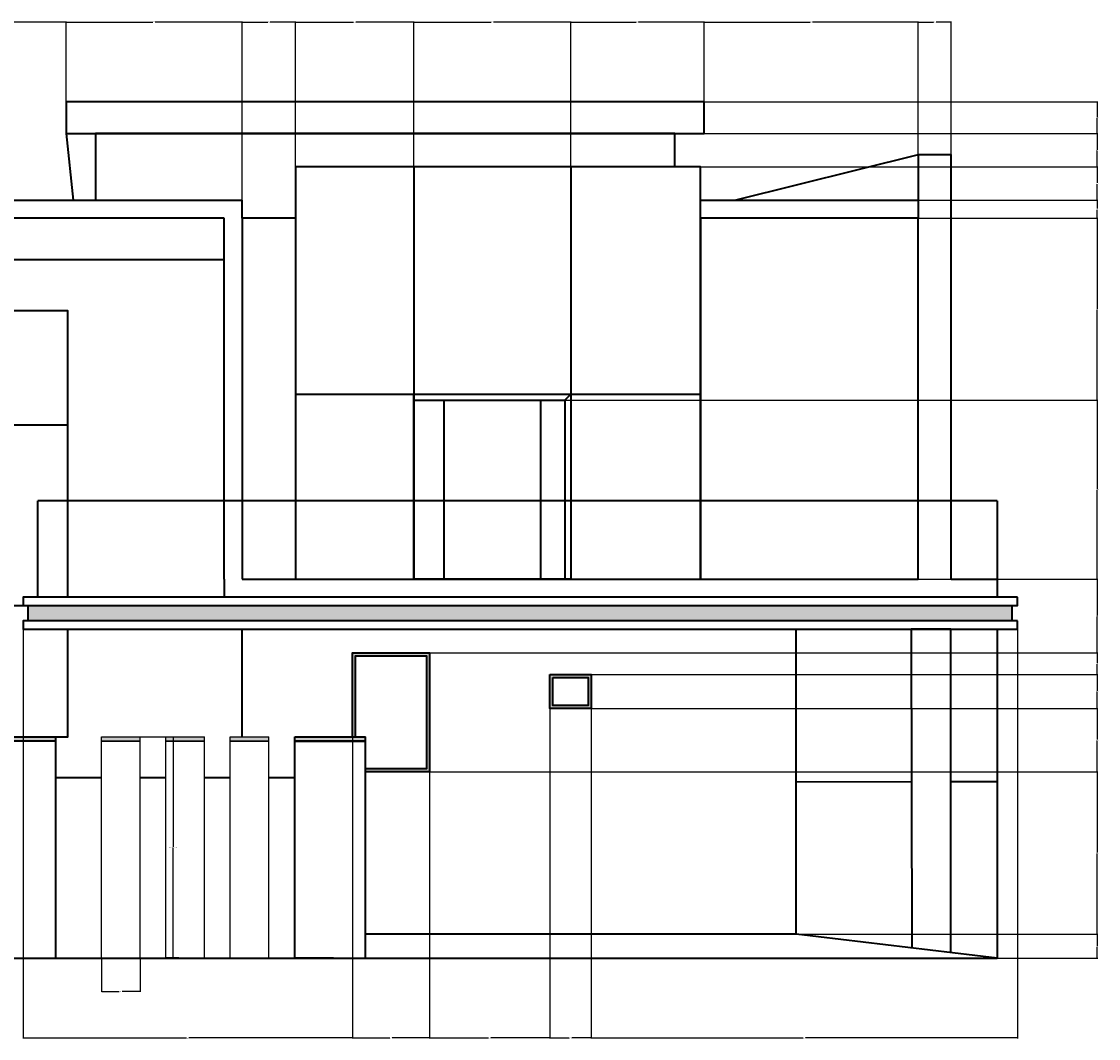
# Model space of a CAD drawing. Units: feet. Extents: x 2651 to 4047, y 949 to 1287.
# Tile 5 of 5: x 3689 to 4047, y 949 to 1287. Entities that reach past the tile are written whole.
import ezdxf

# ---------------------------------------------------------------- set-up
doc = ezdxf.new("R2010")
doc.units = ezdxf.units.FT
for name, color, linetype, lineweight in [('A-ANNO-DIMS', 2, 'Continuous', 18), ('A-ELEV', 7, 'Continuous', 35), ('A-ELEV-FNCE', 7, 'Continuous', 25), ('A-ELEV-PATT', 8, 'Continuous', 13)]:
    doc.layers.add(name, color=color, linetype=linetype, lineweight=lineweight)
doc.styles.get("Standard").update_dxf_attribs({"font": 'arial.ttf'})
doc.dimstyles.get("Standard").update_dxf_attribs({"dimtxt": 0.18, "dimasz": 0.18, "dimexe": 0.18, "dimexo": 0.0625, "dimgap": 0.09, "dimtad": 0, "dimtih": 1, "dimtoh": 1, "dimdec": 1, "dimzin": 0, "dimdsep": 46, "dimlunit": 3, "dimtxsty": 'Standard', "dimcen": 0.09, "dimadec": 0, "dimazin": 0, "dimtfac": 1, "dimtdec": 1, "dimtofl": 0, "dimtmove": 0, "dimatfit": 3, "dimfxl": 1, "dimtolj": 1, "dimtzin": 0, "dimarcsym": 0})

# ---------------------------------------------------------------- blocks, each defined once
blk = doc.blocks.new('BOUNDARY-PIER')
for p, q in [((0, 72.1), (0, 73.54)), ((12.86, 0), (12.86, 73.54))]:
    blk.add_line(p, q)
for points in [[(0, 73.54), (12.86, 73.54)], [(12.86, 0), (0, 0), (0, 72.1), (12.86, 72.1)], [(12.86, 72.1), (0, 72.1)]]:
    blk.add_lwpolyline(points)
blk = doc.blocks.new('*D5')
at = {"layer": 'A-ANNO-DIMS', "color": 0, "lineweight": -2, "transparency": 16777216}
for p, q in [((3728.81, 1049.19), (3739.96, 1049.19)), ((3739.78, 1049.01), (3739.78, 1012.6)), ((3739.78, 975.83), (3739.78, 1012.23)), ((3728.81, 975.65), (3739.96, 975.65))]:
    blk.add_line(p, q, dxfattribs=at)
at = {"layer": 'A-ANNO-DIMS', "color": 0, "transparency": 16777216}
for points in [[(3739.75, 1049.01), (3739.81, 1049.01), (3739.78, 1049.19)], [(3739.75, 975.83), (3739.81, 975.83), (3739.78, 975.65)]]:
    blk.add_solid(points, dxfattribs=at)
at = {"layer": 'Defpoints', "color": 0, "transparency": 16777216}
for p in [(3728.75, 1049.19), (3739.78, 1049.19), (3728.75, 975.65)]:
    blk.add_point(p, dxfattribs=at)
at = {"layer": 'A-ANNO-DIMS', "color": 0, "transparency": 16777216, "insert": (3739.78, 1012.42), "char_height": 0.18, "attachment_point": 5}
blk.add_mtext('\\A1;BOUNDARY PIER 74 TYP.', dxfattribs=at)
blk = doc.blocks.new('*D6')
at = {"layer": 'A-ANNO-DIMS', "color": 0, "lineweight": -2, "transparency": 16777216}
for p, q in [((3715.89, 975.59), (3715.89, 964.44)), ((3728.75, 975.59), (3728.75, 964.44)), ((3716.07, 964.62), (3721.8, 964.62)), ((3728.57, 964.62), (3722.84, 964.62))]:
    blk.add_line(p, q, dxfattribs=at)
at = {"layer": 'A-ANNO-DIMS', "color": 0, "transparency": 16777216}
for points in [[(3716.07, 964.65), (3716.07, 964.59), (3715.89, 964.62)], [(3728.57, 964.65), (3728.57, 964.59), (3728.75, 964.62)]]:
    blk.add_solid(points, dxfattribs=at)
at = {"layer": 'Defpoints', "color": 0, "transparency": 16777216}
for p in [(3715.89, 975.65), (3728.75, 975.65), (3728.75, 964.62)]:
    blk.add_point(p, dxfattribs=at)
at = {"layer": 'A-ANNO-DIMS', "color": 0, "transparency": 16777216, "insert": (3722.32, 964.62), "char_height": 0.18, "attachment_point": 5}
blk.add_mtext('\\A1;13 TYP.', dxfattribs=at)
blk = doc.blocks.new('*D30')
at = {"layer": 'A-ANNO-DIMS', "color": 0, "lineweight": -2, "transparency": 16777216}
for p, q in [((3655.82, 1190.93), (3655.82, 1287.01)), ((3656, 1286.83), (3679.52, 1286.83)), ((3703.97, 1286.83), (3680.45, 1286.83)), ((3704.15, 1260.39), (3704.15, 1287.01))]:
    blk.add_line(p, q, dxfattribs=at)
at = {"layer": 'A-ANNO-DIMS', "color": 0, "transparency": 16777216}
for points in [[(3656, 1286.86), (3656, 1286.8), (3655.82, 1286.83)], [(3703.97, 1286.86), (3703.97, 1286.8), (3704.15, 1286.83)]]:
    blk.add_solid(points, dxfattribs=at)
at = {"layer": 'Defpoints', "color": 0, "transparency": 16777216}
for p in [(3704.15, 1286.83), (3704.15, 1260.33), (3655.82, 1190.87)]:
    blk.add_point(p, dxfattribs=at)
at = {"layer": 'A-ANNO-DIMS', "color": 0, "transparency": 16777216, "insert": (3679.99, 1286.83), "char_height": 0.18, "attachment_point": 5}
blk.add_mtext('\\A1;48.335', dxfattribs=at)
blk = doc.blocks.new('*D31')
at = {"layer": 'A-ANNO-DIMS', "color": 0, "lineweight": -2, "transparency": 16777216}
for p, q in [((3704.15, 1260.39), (3704.15, 1287.01)), ((3704.33, 1286.83), (3733.04, 1286.83)), ((3762.53, 1286.83), (3733.83, 1286.83)), ((3762.71, 1227.71), (3762.71, 1287.01))]:
    blk.add_line(p, q, dxfattribs=at)
at = {"layer": 'A-ANNO-DIMS', "color": 0, "transparency": 16777216}
for points in [[(3704.33, 1286.86), (3704.33, 1286.8), (3704.15, 1286.83)], [(3762.53, 1286.86), (3762.53, 1286.8), (3762.71, 1286.83)]]:
    blk.add_solid(points, dxfattribs=at)
at = {"layer": 'Defpoints', "color": 0, "transparency": 16777216}
for p in [(3762.71, 1286.83), (3704.15, 1260.33), (3762.71, 1227.65)]:
    blk.add_point(p, dxfattribs=at)
at = {"layer": 'A-ANNO-DIMS', "color": 0, "transparency": 16777216, "insert": (3733.43, 1286.83), "char_height": 0.18, "attachment_point": 5}
blk.add_mtext('\\A1;58.56', dxfattribs=at)
blk = doc.blocks.new('*D32')
at = {"layer": 'A-ANNO-DIMS', "color": 0, "lineweight": -2, "transparency": 16777216}
for p, q in [((3762.71, 1227.71), (3762.71, 1287.01)), ((3762.89, 1286.83), (3771.2, 1286.83)), ((3780.27, 1286.83), (3771.97, 1286.83)), ((3780.45, 1238.76), (3780.45, 1287.01))]:
    blk.add_line(p, q, dxfattribs=at)
at = {"layer": 'A-ANNO-DIMS', "color": 0, "transparency": 16777216}
for points in [[(3762.89, 1286.86), (3762.89, 1286.8), (3762.71, 1286.83)], [(3780.27, 1286.86), (3780.27, 1286.8), (3780.45, 1286.83)]]:
    blk.add_solid(points, dxfattribs=at)
at = {"layer": 'Defpoints', "color": 0, "transparency": 16777216}
for p in [(3780.45, 1286.83), (3780.45, 1238.69), (3762.71, 1227.65)]:
    blk.add_point(p, dxfattribs=at)
at = {"layer": 'A-ANNO-DIMS', "color": 0, "transparency": 16777216, "insert": (3771.58, 1286.83), "char_height": 0.18, "attachment_point": 5}
blk.add_mtext('\\A1;17.74', dxfattribs=at)
blk = doc.blocks.new('*D33')
at = {"layer": 'A-ANNO-DIMS', "color": 0, "lineweight": -2, "transparency": 16777216}
for p, q in [((3780.45, 1238.76), (3780.45, 1287.01)), ((3780.63, 1286.83), (3799.7, 1286.83)), ((3819.56, 1286.83), (3800.49, 1286.83)), ((3819.74, 1238.76), (3819.74, 1287.01))]:
    blk.add_line(p, q, dxfattribs=at)
at = {"layer": 'A-ANNO-DIMS', "color": 0, "transparency": 16777216}
for points in [[(3780.63, 1286.86), (3780.63, 1286.8), (3780.45, 1286.83)], [(3819.56, 1286.86), (3819.56, 1286.8), (3819.74, 1286.83)]]:
    blk.add_solid(points, dxfattribs=at)
at = {"layer": 'Defpoints', "color": 0, "transparency": 16777216}
for p in [(3819.74, 1286.83), (3780.45, 1238.69), (3819.74, 1238.69)]:
    blk.add_point(p, dxfattribs=at)
at = {"layer": 'A-ANNO-DIMS', "color": 0, "transparency": 16777216, "insert": (3800.1, 1286.83), "char_height": 0.18, "attachment_point": 5}
blk.add_mtext('\\A1;39.29', dxfattribs=at)
blk = doc.blocks.new('*D34')
at = {"layer": 'A-ANNO-DIMS', "color": 0, "lineweight": -2, "transparency": 16777216}
for p, q in [((3819.74, 1238.76), (3819.74, 1287.01)), ((3819.92, 1286.83), (3845.47, 1286.83)), ((3871.78, 1286.83), (3846.23, 1286.83)), ((3871.96, 1238.76), (3871.96, 1287.01))]:
    blk.add_line(p, q, dxfattribs=at)
at = {"layer": 'A-ANNO-DIMS', "color": 0, "transparency": 16777216}
for points in [[(3819.92, 1286.86), (3819.92, 1286.8), (3819.74, 1286.83)], [(3871.78, 1286.86), (3871.78, 1286.8), (3871.96, 1286.83)]]:
    blk.add_solid(points, dxfattribs=at)
at = {"layer": 'Defpoints', "color": 0, "transparency": 16777216}
for p in [(3871.96, 1286.83), (3819.74, 1238.69), (3871.96, 1238.69)]:
    blk.add_point(p, dxfattribs=at)
at = {"layer": 'A-ANNO-DIMS', "color": 0, "transparency": 16777216, "insert": (3845.85, 1286.83), "char_height": 0.18, "attachment_point": 5}
blk.add_mtext('\\A1;52.21', dxfattribs=at)
blk = doc.blocks.new('*D35')
at = {"layer": 'A-ANNO-DIMS', "color": 0, "lineweight": -2, "transparency": 16777216}
for p, q in [((3871.96, 1238.76), (3871.96, 1287.01)), ((3872.14, 1286.83), (3893.73, 1286.83)), ((3916.09, 1286.83), (3894.49, 1286.83)), ((3916.27, 1260.39), (3916.27, 1287.01))]:
    blk.add_line(p, q, dxfattribs=at)
at = {"layer": 'A-ANNO-DIMS', "color": 0, "transparency": 16777216}
for points in [[(3872.14, 1286.86), (3872.14, 1286.8), (3871.96, 1286.83)], [(3916.09, 1286.86), (3916.09, 1286.8), (3916.27, 1286.83)]]:
    blk.add_solid(points, dxfattribs=at)
at = {"layer": 'Defpoints', "color": 0, "transparency": 16777216}
for p in [(3916.27, 1286.83), (3916.27, 1260.33), (3871.96, 1238.69)]:
    blk.add_point(p, dxfattribs=at)
at = {"layer": 'A-ANNO-DIMS', "color": 0, "transparency": 16777216, "insert": (3894.11, 1286.83), "char_height": 0.18, "attachment_point": 5}
blk.add_mtext('\\A1;44.31', dxfattribs=at)
blk = doc.blocks.new('*D36')
at = {"layer": 'A-ANNO-DIMS', "color": 0, "lineweight": -2, "transparency": 16777216}
for p, q in [((3916.27, 1260.39), (3916.27, 1287.01)), ((3916.45, 1286.83), (3951.5, 1286.83)), ((3987.3, 1286.83), (3952.25, 1286.83)), ((3987.48, 1242.75), (3987.48, 1287.01))]:
    blk.add_line(p, q, dxfattribs=at)
at = {"layer": 'A-ANNO-DIMS', "color": 0, "transparency": 16777216}
for points in [[(3916.45, 1286.86), (3916.45, 1286.8), (3916.27, 1286.83)], [(3987.3, 1286.86), (3987.3, 1286.8), (3987.48, 1286.83)]]:
    blk.add_solid(points, dxfattribs=at)
at = {"layer": 'Defpoints', "color": 0, "transparency": 16777216}
for p in [(3987.48, 1286.83), (3916.27, 1260.33), (3987.48, 1242.69)]:
    blk.add_point(p, dxfattribs=at)
at = {"layer": 'A-ANNO-DIMS', "color": 0, "transparency": 16777216, "insert": (3951.87, 1286.83), "char_height": 0.18, "attachment_point": 5}
blk.add_mtext('\\A1;71.21', dxfattribs=at)
blk = doc.blocks.new('*D37')
at = {"layer": 'A-ANNO-DIMS', "color": 0, "lineweight": -2, "transparency": 16777216}
for p, q in [((3987.48, 1242.75), (3987.48, 1287.01)), ((3987.66, 1286.83), (3992.49, 1286.83)), ((3998.23, 1286.83), (3993.4, 1286.83)), ((3998.41, 1242.75), (3998.41, 1287.01))]:
    blk.add_line(p, q, dxfattribs=at)
at = {"layer": 'A-ANNO-DIMS', "color": 0, "transparency": 16777216}
for points in [[(3987.66, 1286.86), (3987.66, 1286.8), (3987.48, 1286.83)], [(3998.23, 1286.86), (3998.23, 1286.8), (3998.41, 1286.83)]]:
    blk.add_solid(points, dxfattribs=at)
at = {"layer": 'Defpoints', "color": 0, "transparency": 16777216}
for p in [(3998.41, 1286.83), (3987.48, 1242.69), (3998.41, 1242.69)]:
    blk.add_point(p, dxfattribs=at)
at = {"layer": 'A-ANNO-DIMS', "color": 0, "transparency": 16777216, "insert": (3992.95, 1286.83), "char_height": 0.18, "attachment_point": 5}
blk.add_mtext('\\A1;10.936', dxfattribs=at)
blk = doc.blocks.new('*D38')
at = {"layer": 'A-ANNO-DIMS', "color": 0, "lineweight": -2, "transparency": 16777216}
for p, q in [((3689.92, 1084.91), (3689.92, 948.97)), ((3799.33, 1077.11), (3799.33, 948.97)), ((3690.1, 949.15), (3744.24, 949.15)), ((3799.15, 949.15), (3745.01, 949.15))]:
    blk.add_line(p, q, dxfattribs=at)
at = {"layer": 'A-ANNO-DIMS', "color": 0, "transparency": 16777216}
for points in [[(3690.1, 949.18), (3690.1, 949.12), (3689.92, 949.15)], [(3799.15, 949.18), (3799.15, 949.12), (3799.33, 949.15)]]:
    blk.add_solid(points, dxfattribs=at)
at = {"layer": 'Defpoints', "color": 0, "transparency": 16777216}
for p in [(3689.92, 1084.98), (3799.33, 1077.18), (3799.33, 949.15)]:
    blk.add_point(p, dxfattribs=at)
at = {"layer": 'A-ANNO-DIMS', "color": 0, "transparency": 16777216, "insert": (3744.62, 949.15), "char_height": 0.18, "attachment_point": 5}
blk.add_mtext('\\A1;109.4', dxfattribs=at)
blk = doc.blocks.new('*D39')
at = {"layer": 'A-ANNO-DIMS', "color": 0, "lineweight": -2, "transparency": 16777216}
for p, q in [((3799.33, 1077.11), (3799.33, 948.97)), ((3825, 1077.11), (3825, 948.97)), ((3799.51, 949.15), (3811.77, 949.15)), ((3824.82, 949.15), (3812.56, 949.15))]:
    blk.add_line(p, q, dxfattribs=at)
at = {"layer": 'A-ANNO-DIMS', "color": 0, "transparency": 16777216}
for points in [[(3799.51, 949.18), (3799.51, 949.12), (3799.33, 949.15)], [(3824.82, 949.18), (3824.82, 949.12), (3825, 949.15)]]:
    blk.add_solid(points, dxfattribs=at)
at = {"layer": 'Defpoints', "color": 0, "transparency": 16777216}
for p in [(3799.33, 1077.18), (3825, 1077.18), (3825, 949.15)]:
    blk.add_point(p, dxfattribs=at)
at = {"layer": 'A-ANNO-DIMS', "color": 0, "transparency": 16777216, "insert": (3812.16, 949.15), "char_height": 0.18, "attachment_point": 5}
blk.add_mtext('\\A1;25.67', dxfattribs=at)
blk = doc.blocks.new('*D40')
at = {"layer": 'A-ANNO-DIMS', "color": 0, "lineweight": -2, "transparency": 16777216}
for p, q in [((3825, 1077.11), (3825, 948.97)), ((3865.03, 1069.91), (3865.03, 948.97)), ((3825.18, 949.15), (3844.62, 949.15)), ((3864.85, 949.15), (3845.41, 949.15))]:
    blk.add_line(p, q, dxfattribs=at)
at = {"layer": 'A-ANNO-DIMS', "color": 0, "transparency": 16777216}
for points in [[(3825.18, 949.18), (3825.18, 949.12), (3825, 949.15)], [(3864.85, 949.18), (3864.85, 949.12), (3865.03, 949.15)]]:
    blk.add_solid(points, dxfattribs=at)
at = {"layer": 'Defpoints', "color": 0, "transparency": 16777216}
for p in [(3825, 1077.18), (3865.03, 1069.98), (3865.03, 949.15)]:
    blk.add_point(p, dxfattribs=at)
at = {"layer": 'A-ANNO-DIMS', "color": 0, "transparency": 16777216, "insert": (3845.01, 949.15), "char_height": 0.18, "attachment_point": 5}
blk.add_mtext('\\A1;40.03', dxfattribs=at)
blk = doc.blocks.new('*D41')
at = {"layer": 'A-ANNO-DIMS', "color": 0, "lineweight": -2, "transparency": 16777216}
for p, q in [((3865.03, 1069.91), (3865.03, 948.97)), ((3878.69, 1069.91), (3878.69, 948.97)), ((3865.21, 949.15), (3871.41, 949.15)), ((3878.51, 949.15), (3872.32, 949.15))]:
    blk.add_line(p, q, dxfattribs=at)
at = {"layer": 'A-ANNO-DIMS', "color": 0, "transparency": 16777216}
for points in [[(3865.21, 949.18), (3865.21, 949.12), (3865.03, 949.15)], [(3878.51, 949.18), (3878.51, 949.12), (3878.69, 949.15)]]:
    blk.add_solid(points, dxfattribs=at)
at = {"layer": 'Defpoints', "color": 0, "transparency": 16777216}
for p in [(3865.03, 1069.98), (3878.69, 1069.98), (3878.69, 949.15)]:
    blk.add_point(p, dxfattribs=at)
at = {"layer": 'A-ANNO-DIMS', "color": 0, "transparency": 16777216, "insert": (3871.86, 949.15), "char_height": 0.18, "attachment_point": 5}
blk.add_mtext('\\A1;13.666', dxfattribs=at)
blk = doc.blocks.new('*D42')
at = {"layer": 'A-ANNO-DIMS', "color": 0, "lineweight": -2, "transparency": 16777216}
for p, q in [((4020.49, 1084.91), (4020.49, 948.97)), ((3878.69, 1069.91), (3878.69, 948.97)), ((3878.87, 949.15), (3949.21, 949.15)), ((4020.31, 949.15), (3949.98, 949.15))]:
    blk.add_line(p, q, dxfattribs=at)
at = {"layer": 'A-ANNO-DIMS', "color": 0, "transparency": 16777216}
for points in [[(3878.87, 949.18), (3878.87, 949.12), (3878.69, 949.15)], [(4020.31, 949.18), (4020.31, 949.12), (4020.49, 949.15)]]:
    blk.add_solid(points, dxfattribs=at)
at = {"layer": 'Defpoints', "color": 0, "transparency": 16777216}
for p in [(4020.49, 1084.98), (3878.69, 1069.98), (4020.49, 949.15)]:
    blk.add_point(p, dxfattribs=at)
at = {"layer": 'A-ANNO-DIMS', "color": 0, "transparency": 16777216, "insert": (3949.59, 949.15), "char_height": 0.18, "attachment_point": 5}
blk.add_mtext('\\A1;141.8', dxfattribs=at)
blk = doc.blocks.new('*D54')
at = {"layer": 'A-ANNO-DIMS', "color": 0, "lineweight": -2, "transparency": 16777216}
for p, q in [((3946.94, 983.61), (4047.17, 983.61)), ((4046.99, 983.43), (4046.99, 979.81)), ((4046.99, 975.83), (4046.99, 979.45)), ((4013.79, 975.65), (4047.17, 975.65))]:
    blk.add_line(p, q, dxfattribs=at)
at = {"layer": 'A-ANNO-DIMS', "color": 0, "transparency": 16777216}
for points in [[(4046.96, 983.43), (4047.02, 983.43), (4046.99, 983.61)], [(4046.96, 975.83), (4047.02, 975.83), (4046.99, 975.65)]]:
    blk.add_solid(points, dxfattribs=at)
at = {"layer": 'Defpoints', "color": 0, "transparency": 16777216}
for p in [(3946.87, 983.61), (4046.99, 983.61), (4013.73, 975.65)]:
    blk.add_point(p, dxfattribs=at)
at = {"layer": 'A-ANNO-DIMS', "color": 0, "transparency": 16777216, "insert": (4046.99, 979.63), "char_height": 0.18, "attachment_point": 5}
blk.add_mtext('\\A1;7.961', dxfattribs=at)
blk = doc.blocks.new('*D55')
at = {"layer": 'A-ANNO-DIMS', "color": 0, "lineweight": -2, "transparency": 16777216}
for p, q in [((3825.06, 1037.57), (4047.17, 1037.57)), ((4046.99, 1037.39), (4046.99, 1010.77)), ((4046.99, 983.79), (4046.99, 1010.41)), ((3946.94, 983.61), (4047.17, 983.61))]:
    blk.add_line(p, q, dxfattribs=at)
at = {"layer": 'A-ANNO-DIMS', "color": 0, "transparency": 16777216}
for points in [[(4046.96, 1037.39), (4047.02, 1037.39), (4046.99, 1037.57)], [(4046.96, 983.79), (4047.02, 983.79), (4046.99, 983.61)]]:
    blk.add_solid(points, dxfattribs=at)
at = {"layer": 'Defpoints', "color": 0, "transparency": 16777216}
for p in [(3825, 1037.57), (4046.99, 1037.57), (3946.87, 983.61)]:
    blk.add_point(p, dxfattribs=at)
at = {"layer": 'A-ANNO-DIMS', "color": 0, "transparency": 16777216, "insert": (4046.99, 1010.59), "char_height": 0.18, "attachment_point": 5}
blk.add_mtext('\\A1;53.96', dxfattribs=at)
blk = doc.blocks.new('*D56')
at = {"layer": 'A-ANNO-DIMS', "color": 0, "lineweight": -2, "transparency": 16777216}
for p, q in [((3878.76, 1058.68), (4047.17, 1058.68)), ((4046.99, 1058.5), (4046.99, 1048.31)), ((4046.99, 1037.75), (4046.99, 1047.94)), ((3825.06, 1037.57), (4047.17, 1037.57))]:
    blk.add_line(p, q, dxfattribs=at)
at = {"layer": 'A-ANNO-DIMS', "color": 0, "transparency": 16777216}
for points in [[(4046.96, 1058.5), (4047.02, 1058.5), (4046.99, 1058.68)], [(4046.96, 1037.75), (4047.02, 1037.75), (4046.99, 1037.57)]]:
    blk.add_solid(points, dxfattribs=at)
at = {"layer": 'Defpoints', "color": 0, "transparency": 16777216}
for p in [(3878.69, 1058.68), (4046.99, 1058.68), (3825, 1037.57)]:
    blk.add_point(p, dxfattribs=at)
at = {"layer": 'A-ANNO-DIMS', "color": 0, "transparency": 16777216, "insert": (4046.99, 1048.12), "char_height": 0.18, "attachment_point": 5}
blk.add_mtext('\\A1;21.114', dxfattribs=at)
blk = doc.blocks.new('*D57')
at = {"layer": 'A-ANNO-DIMS', "color": 0, "lineweight": -2, "transparency": 16777216}
for p, q in [((3878.76, 1069.98), (4047.17, 1069.98)), ((4046.99, 1069.8), (4046.99, 1064.51)), ((4046.99, 1058.86), (4046.99, 1064.15)), ((3878.76, 1058.68), (4047.17, 1058.68))]:
    blk.add_line(p, q, dxfattribs=at)
at = {"layer": 'A-ANNO-DIMS', "color": 0, "transparency": 16777216}
for points in [[(4046.96, 1069.8), (4047.02, 1069.8), (4046.99, 1069.98)], [(4046.96, 1058.86), (4047.02, 1058.86), (4046.99, 1058.68)]]:
    blk.add_solid(points, dxfattribs=at)
at = {"layer": 'Defpoints', "color": 0, "transparency": 16777216}
for p in [(3878.69, 1069.98), (4046.99, 1069.98), (3878.69, 1058.68)]:
    blk.add_point(p, dxfattribs=at)
at = {"layer": 'A-ANNO-DIMS', "color": 0, "transparency": 16777216, "insert": (4046.99, 1064.33), "char_height": 0.18, "attachment_point": 5}
blk.add_mtext('\\A1;11.295', dxfattribs=at)
blk = doc.blocks.new('*D58')
at = {"layer": 'A-ANNO-DIMS', "color": 0, "lineweight": -2, "transparency": 16777216}
for p, q in [((3825.06, 1077.18), (4047.17, 1077.18)), ((4046.99, 1077), (4046.99, 1073.76)), ((4046.99, 1070.16), (4046.99, 1073.4)), ((3878.76, 1069.98), (4047.17, 1069.98))]:
    blk.add_line(p, q, dxfattribs=at)
at = {"layer": 'A-ANNO-DIMS', "color": 0, "transparency": 16777216}
for points in [[(4046.96, 1077), (4047.02, 1077), (4046.99, 1077.18)], [(4046.96, 1070.16), (4047.02, 1070.16), (4046.99, 1069.98)]]:
    blk.add_solid(points, dxfattribs=at)
at = {"layer": 'Defpoints', "color": 0, "transparency": 16777216}
for p in [(3825, 1077.18), (4046.99, 1077.18), (3878.69, 1069.98)]:
    blk.add_point(p, dxfattribs=at)
at = {"layer": 'A-ANNO-DIMS', "color": 0, "transparency": 16777216, "insert": (4046.99, 1073.58), "char_height": 0.18, "attachment_point": 5}
blk.add_mtext('\\A1;7.2', dxfattribs=at)
blk = doc.blocks.new('*D59')
at = {"layer": 'A-ANNO-DIMS', "color": 0, "lineweight": -2, "transparency": 16777216}
for p, q in [((3872.02, 1101.65), (4047.17, 1101.65)), ((4046.99, 1101.47), (4046.99, 1089.59)), ((4046.99, 1077.36), (4046.99, 1089.23)), ((3825.06, 1077.18), (4047.17, 1077.18))]:
    blk.add_line(p, q, dxfattribs=at)
at = {"layer": 'A-ANNO-DIMS', "color": 0, "transparency": 16777216}
for points in [[(4046.96, 1101.47), (4047.02, 1101.47), (4046.99, 1101.65)], [(4046.96, 1077.36), (4047.02, 1077.36), (4046.99, 1077.18)]]:
    blk.add_solid(points, dxfattribs=at)
at = {"layer": 'Defpoints', "color": 0, "transparency": 16777216}
for p in [(3871.96, 1101.65), (4046.99, 1101.65), (3825, 1077.18)]:
    blk.add_point(p, dxfattribs=at)
at = {"layer": 'A-ANNO-DIMS', "color": 0, "transparency": 16777216, "insert": (4046.99, 1089.41), "char_height": 0.18, "attachment_point": 5}
blk.add_mtext('\\A1;24.474', dxfattribs=at)
blk = doc.blocks.new('*D60')
at = {"layer": 'A-ANNO-DIMS', "color": 0, "lineweight": -2, "transparency": 16777216}
for p, q in [((3870.02, 1161.11), (4047.17, 1161.11)), ((4046.99, 1160.93), (4046.99, 1131.56)), ((4046.99, 1101.83), (4046.99, 1131.2)), ((3872.02, 1101.65), (4047.17, 1101.65))]:
    blk.add_line(p, q, dxfattribs=at)
at = {"layer": 'A-ANNO-DIMS', "color": 0, "transparency": 16777216}
for points in [[(4046.96, 1160.93), (4047.02, 1160.93), (4046.99, 1161.11)], [(4046.96, 1101.83), (4047.02, 1101.83), (4046.99, 1101.65)]]:
    blk.add_solid(points, dxfattribs=at)
at = {"layer": 'Defpoints', "color": 0, "transparency": 16777216}
for p in [(3869.96, 1161.11), (4046.99, 1161.11), (3871.96, 1101.65)]:
    blk.add_point(p, dxfattribs=at)
at = {"layer": 'A-ANNO-DIMS', "color": 0, "transparency": 16777216, "insert": (4046.99, 1131.38), "char_height": 0.18, "attachment_point": 5}
blk.add_mtext('\\A1;59.46', dxfattribs=at)
blk = doc.blocks.new('*D61')
at = {"layer": 'A-ANNO-DIMS', "color": 0, "lineweight": -2, "transparency": 16777216}
for p, q in [((3987.54, 1221.65), (4047.17, 1221.65)), ((4046.99, 1221.47), (4046.99, 1191.56)), ((4046.99, 1161.29), (4046.99, 1191.2)), ((3870.02, 1161.11), (4047.17, 1161.11))]:
    blk.add_line(p, q, dxfattribs=at)
at = {"layer": 'A-ANNO-DIMS', "color": 0, "transparency": 16777216}
for points in [[(4046.96, 1221.47), (4047.02, 1221.47), (4046.99, 1221.65)], [(4046.96, 1161.29), (4047.02, 1161.29), (4046.99, 1161.11)]]:
    blk.add_solid(points, dxfattribs=at)
at = {"layer": 'Defpoints', "color": 0, "transparency": 16777216}
for p in [(3987.48, 1221.65), (4046.99, 1221.65), (3869.96, 1161.11)]:
    blk.add_point(p, dxfattribs=at)
at = {"layer": 'A-ANNO-DIMS', "color": 0, "transparency": 16777216, "insert": (4046.99, 1191.38), "char_height": 0.18, "attachment_point": 5}
blk.add_mtext('\\A1;60.54', dxfattribs=at)
blk = doc.blocks.new('*D62')
at = {"layer": 'A-ANNO-DIMS', "color": 0, "lineweight": -2, "transparency": 16777216}
for p, q in [((3987.54, 1227.65), (4047.17, 1227.65)), ((4046.99, 1227.47), (4046.99, 1224.83)), ((4046.99, 1221.83), (4046.99, 1224.47)), ((3987.54, 1221.65), (4047.17, 1221.65))]:
    blk.add_line(p, q, dxfattribs=at)
at = {"layer": 'A-ANNO-DIMS', "color": 0, "transparency": 16777216}
for points in [[(4046.96, 1227.47), (4047.02, 1227.47), (4046.99, 1227.65)], [(4046.96, 1221.83), (4047.02, 1221.83), (4046.99, 1221.65)]]:
    blk.add_solid(points, dxfattribs=at)
at = {"layer": 'Defpoints', "color": 0, "transparency": 16777216}
for p in [(3987.48, 1227.65), (4046.99, 1227.65), (3987.48, 1221.65)]:
    blk.add_point(p, dxfattribs=at)
at = {"layer": 'A-ANNO-DIMS', "color": 0, "transparency": 16777216, "insert": (4046.99, 1224.65), "char_height": 0.18, "attachment_point": 5}
blk.add_mtext('\\A1;6', dxfattribs=at)
blk = doc.blocks.new('*D63')
at = {"layer": 'A-ANNO-DIMS', "color": 0, "lineweight": -2, "transparency": 16777216}
for p, q in [((3780.52, 1238.69), (4047.17, 1238.69)), ((4046.99, 1238.51), (4046.99, 1233.35)), ((4046.99, 1227.83), (4046.99, 1232.99)), ((3987.54, 1227.65), (4047.17, 1227.65))]:
    blk.add_line(p, q, dxfattribs=at)
at = {"layer": 'A-ANNO-DIMS', "color": 0, "transparency": 16777216}
for points in [[(4046.96, 1238.51), (4047.02, 1238.51), (4046.99, 1238.69)], [(4046.96, 1227.83), (4047.02, 1227.83), (4046.99, 1227.65)]]:
    blk.add_solid(points, dxfattribs=at)
at = {"layer": 'Defpoints', "color": 0, "transparency": 16777216}
for p in [(3780.45, 1238.69), (4046.99, 1238.69), (3987.48, 1227.65)]:
    blk.add_point(p, dxfattribs=at)
at = {"layer": 'A-ANNO-DIMS', "color": 0, "transparency": 16777216, "insert": (4046.99, 1233.17), "char_height": 0.18, "attachment_point": 5}
blk.add_mtext('\\A1;11.044', dxfattribs=at)
blk = doc.blocks.new('*D64')
at = {"layer": 'A-ANNO-DIMS', "color": 0, "lineweight": -2, "transparency": 16777216}
for p, q in [((3704.22, 1249.74), (4047.17, 1249.74)), ((4046.99, 1249.56), (4046.99, 1244.4)), ((4046.99, 1238.87), (4046.99, 1244.03)), ((3780.52, 1238.69), (4047.17, 1238.69))]:
    blk.add_line(p, q, dxfattribs=at)
at = {"layer": 'A-ANNO-DIMS', "color": 0, "transparency": 16777216}
for points in [[(4046.96, 1249.56), (4047.02, 1249.56), (4046.99, 1249.74)], [(4046.96, 1238.87), (4047.02, 1238.87), (4046.99, 1238.69)]]:
    blk.add_solid(points, dxfattribs=at)
at = {"layer": 'Defpoints', "color": 0, "transparency": 16777216}
for p in [(3704.15, 1249.74), (4046.99, 1249.74), (3780.45, 1238.69)]:
    blk.add_point(p, dxfattribs=at)
at = {"layer": 'A-ANNO-DIMS', "color": 0, "transparency": 16777216, "insert": (4046.99, 1244.22), "char_height": 0.18, "attachment_point": 5}
blk.add_mtext('\\A1;11.044', dxfattribs=at)
blk = doc.blocks.new('*D65')
at = {"layer": 'A-ANNO-DIMS', "color": 0, "lineweight": -2, "transparency": 16777216}
for p, q in [((3704.22, 1260.33), (4047.17, 1260.33)), ((4046.99, 1260.15), (4046.99, 1255.22)), ((4046.99, 1249.92), (4046.99, 1254.85)), ((3704.22, 1249.74), (4047.17, 1249.74))]:
    blk.add_line(p, q, dxfattribs=at)
at = {"layer": 'A-ANNO-DIMS', "color": 0, "transparency": 16777216}
for points in [[(4046.96, 1260.15), (4047.02, 1260.15), (4046.99, 1260.33)], [(4046.96, 1249.92), (4047.02, 1249.92), (4046.99, 1249.74)]]:
    blk.add_solid(points, dxfattribs=at)
at = {"layer": 'Defpoints', "color": 0, "transparency": 16777216}
for p in [(3704.15, 1260.33), (4046.99, 1260.33), (3704.15, 1249.74)]:
    blk.add_point(p, dxfattribs=at)
at = {"layer": 'A-ANNO-DIMS', "color": 0, "transparency": 16777216, "insert": (4046.99, 1255.03), "char_height": 0.18, "attachment_point": 5}
blk.add_mtext('\\A1;10.592', dxfattribs=at)

msp = doc.modelspace()

# ---------------------------------------------------------------- hatches: boundary and pattern name
at = {"layer": 'A-ELEV-PATT'}
h = msp.add_hatch(color=256, dxfattribs=at)
h.paths.add_polyline_path([(3655.8177, 1148.4143), (3581.2486, 1148.4143), (3581.2486, 1099.175), (3655.8177, 1099.175)])
h.paths.add_polyline_path([(3653.8177, 1146.4143), (3653.8177, 1101.175), (3583.2486, 1101.175), (3583.2486, 1146.4143)], flags=16)
h.paths.add_polyline_path([(3637.4637, 1135.9058), (3637.4637, 1113.3773), (3599.831, 1113.3773), (3599.831, 1135.9058)], flags=0)
h.paths.add_polyline_path([(3636.8563, 1135.3515), (3636.8563, 1113.9316), (3600.4385, 1113.9316), (3600.4385, 1135.3515)], flags=0)
h.paths.add_polyline_path([(3600.4385, 1146.4143), (3599.831, 1146.4143), (3599.831, 1135.9058), (3600.4385, 1135.9058)], flags=0)
h.paths.add_polyline_path([(3599.831, 1135.9058), (3583.2486, 1135.9058), (3583.2486, 1135.3515), (3599.831, 1135.3515)], flags=0)
h.paths.add_polyline_path([(3653.8177, 1135.9058), (3637.4637, 1135.9058), (3637.4637, 1135.3515), (3653.8177, 1135.3515)], flags=0)
h.paths.add_polyline_path([(3637.4637, 1146.4143), (3636.8563, 1146.4143), (3636.8563, 1135.9058), (3637.4637, 1135.9058)], flags=0)
h.paths.add_polyline_path([(3653.8177, 1113.9316), (3637.4637, 1113.9316), (3637.4637, 1113.3773), (3653.8177, 1113.3773)], flags=0)
h.paths.add_polyline_path([(3637.4637, 1113.3773), (3636.8563, 1113.3773), (3636.8563, 1101.175), (3637.4637, 1101.175)], flags=0)
h.paths.add_polyline_path([(3599.831, 1113.9316), (3583.2486, 1113.9316), (3583.2486, 1113.3773), (3599.831, 1113.3773)], flags=0)
h.paths.add_polyline_path([(3600.4385, 1113.3773), (3599.831, 1113.3773), (3599.831, 1101.175), (3600.4385, 1101.175)], flags=0)
h.paths.add_polyline_path([(3599.4385, 1061.2489), (3598.831, 1061.2489), (3598.831, 1060.6946), (3599.4385, 1060.6946)])
h.paths.add_polyline_path([(3599.4385, 1072.7574), (3598.831, 1072.7574), (3598.831, 1061.2489), (3599.4385, 1061.2489)])
h.paths.add_polyline_path([(3655.8177, 1061.2489), (3599.4385, 1061.2489), (3599.4385, 1060.6946), (3655.8177, 1060.6946)])
h.paths.add_polyline_path([(3598.831, 1061.2489), (3581.2486, 1061.2489), (3581.2486, 1060.6946), (3598.831, 1060.6946)])
h.paths.add_polyline_path([(3599.4385, 1060.6946), (3598.831, 1060.6946), (3598.831, 1049.1862), (3599.4385, 1049.1862)])
h.paths.add_polyline_path([(3598.831, 1072.7574), (3581.2486, 1072.7574), (3581.2486, 1061.2489), (3582.2486, 1061.2489), (3582.2486, 1071.7574), (3598.831, 1071.7574)])
h.paths.add_polyline_path([(3655.8177, 1072.7574), (3599.4385, 1072.7574), (3599.4385, 1071.7574), (3654.8177, 1071.7574), (3654.8177, 1061.2489), (3655.8177, 1061.2489)])
h.paths.add_polyline_path([(3655.8177, 1060.6946), (3654.8177, 1060.6946), (3654.8177, 1050.1862), (3599.4385, 1050.1862), (3599.4385, 1049.1862), (3655.8177, 1049.1862)])
h.paths.add_polyline_path([(3582.2486, 1060.6946), (3581.2486, 1060.6946), (3581.2486, 1049.1862), (3598.831, 1049.1862), (3598.831, 1050.1862), (3582.2486, 1050.1862)])
h.paths.add_polyline_path([(3636.4637, 1071.7574), (3635.8563, 1071.7574), (3635.8563, 1061.2489), (3636.4637, 1061.2489)], flags=17)
h.paths.add_polyline_path([(3636.4637, 1060.6946), (3635.8563, 1060.6946), (3635.8563, 1050.1862), (3636.4637, 1050.1862)], flags=17)
h.paths.add_polyline_path([(3700.7838, 1049.1862), (3536.8233, 1049.1862), (3495.2762, 1049.1862), (3495.2762, 1047.7503), (3700.7838, 1047.7503)])
h.paths.add_polyline_path([(3728.7466, 1049.1862), (3715.891, 1049.1862), (3715.891, 1047.7503), (3728.7466, 1047.7503)])
h.paths.add_polyline_path([(3750.1785, 1049.1862), (3737.323, 1049.1862), (3737.323, 1047.7503), (3750.1785, 1047.7503)])
h.paths.add_polyline_path([(3771.6104, 1049.1862), (3758.7549, 1049.1862), (3758.7549, 1047.7503), (3771.6104, 1047.7503)])
h.paths.add_polyline_path([(3803.7115, 1049.1862), (3780.1868, 1049.1862), (3780.1868, 1047.7503), (3803.7115, 1047.7503)])
h.paths.add_polyline_path([(3824.9977, 1077.1763), (3799.3274, 1077.1763), (3799.3274, 1049.1862), (3800.3274, 1049.1862), (3800.3274, 1076.1763), (3823.9977, 1076.1763), (3823.9977, 1038.5677), (3803.7115, 1038.5677), (3803.7115, 1037.5677), (3824.9977, 1037.5677)])
h.paths.add_polyline_path([(3878.6944, 1069.9768), (3865.0283, 1069.9768), (3865.0283, 1058.6821), (3878.6944, 1058.6821)])
h.paths.add_polyline_path([(3877.6944, 1068.9768), (3877.6944, 1059.6821), (3866.0283, 1059.6821), (3866.0283, 1068.9768)], flags=16)
h = msp.add_hatch(color=256, dxfattribs=at)
h.paths.add_polyline_path([(3655.8177, 1098.3392), (3581.2486, 1098.3392), (3581.2486, 1093.6891), (3655.8177, 1093.6891)])
h.paths.add_polyline_path([(4018.604, 1092.8533), (3691.5404, 1092.8533), (3691.5404, 1087.7738), (4018.604, 1087.7738)])

# ---------------------------------------------------------------- linework, layer by layer
at = {"layer": 'A-ELEV'}
for p, q in [((3704.1528, 1249.7387), (3706.4928, 1227.65)), ((3987.4782, 1242.6921), (3926.8374, 1227.65)), ((3819.7424, 1238.6943), (3819.7424, 1101.65)), ((3871.9572, 1238.6943), (3871.9572, 1101.65)), ((3525.0707, 1227.65), (3762.7135, 1227.65)), ((3762.7135, 1221.65), (3762.7135, 1227.65)), ((3915.0765, 1227.65), (3987.4782, 1227.65)), ((3756.7135, 1221.65), (3525.0707, 1221.65)), ((3780.4541, 1221.65), (3762.7135, 1221.65)), ((3987.4782, 1221.65), (3915.0765, 1221.65)), ((3549.7844, 1207.954), (3756.7135, 1207.954)), ((3780.4541, 1163.1131), (3915.0765, 1163.1131)), ((3829.7716, 1161.1131), (3829.7716, 1101.65)), ((3861.928, 1161.1131), (3861.928, 1101.65)), ((3869.9572, 1161.1131), (3871.9572, 1163.1131)), ((3536.8233, 1152.9072), (3704.7437, 1152.9072)), ((4013.7286, 1127.711), (3694.7424, 1127.711)), ((3694.7424, 1095.65), (3694.7424, 1127.711)), ((4013.7286, 1127.711), (4013.7286, 1095.65)), ((3756.7135, 1101.65), (3756.7135, 1095.65)), ((3762.7135, 1101.65), (3987.4782, 1101.65)), ((3998.4145, 1101.65), (4013.7286, 1101.65)), ((4013.7286, 1095.65), (3704.7437, 1095.65)), ((3536.8233, 1092.8533), (3704.7437, 1092.8533)), ((3762.7135, 1049.1862), (3762.7135, 1084.9772)), ((3946.8725, 983.6108), (3946.8725, 1084.9772)), ((3998.2621, 1084.9772), (3985.0737, 1084.9772)), ((3985.0737, 1084.9772), (3985.2956, 979.0356)), ((3998.2621, 977.4916), (3998.2621, 1084.9772)), ((4013.7286, 1084.9772), (4013.7286, 975.65)), ((3700.7838, 1047.7503), (3700.7838, 1049.1862)), ((3780.1868, 1047.7503), (3780.1868, 1049.1862)), ((3803.7115, 975.65), (3803.7115, 1049.1862)), ((3700.7838, 1035.7503), (3715.891, 1035.7503)), ((3728.7466, 1035.7503), (3737.323, 1035.7503)), ((3750.1785, 1035.7503), (3758.7549, 1035.7503)), ((3771.6104, 1035.7503), (3780.1868, 1035.7503)), ((3946.8725, 1034.294), (3985.1797, 1034.3743)), ((3998.2621, 1034.3743), (4013.7286, 1034.3743)), ((3946.8725, 983.6108), (3803.7115, 983.6108)), ((4013.7286, 975.65), (3946.8725, 983.6108)), ((3495.2762, 975.65), (4013.7286, 975.65))]:
    msp.add_line(p, q, dxfattribs=at)
for points in [[(3704.1528, 1249.7387), (3916.2652, 1249.7387), (3916.2652, 1260.331), (3704.1528, 1260.331)], [(3915.0765, 1101.65), (3987.4782, 1101.65), (3987.4782, 1221.65), (3915.0765, 1221.65)], [(3871.9572, 1101.65), (3819.7424, 1101.65), (3819.7424, 1163.1131), (3871.9572, 1163.1131)], [(4020.4941, 1095.65), (3689.9173, 1095.65), (3689.9173, 1092.8533), (4020.4941, 1092.8533)], [(3691.5404, 1092.8533), (4018.604, 1092.8533), (4018.604, 1087.7738), (3691.5404, 1087.7738)], [(4020.4941, 1087.7738), (3689.9173, 1087.7738), (3689.9173, 1084.9772), (4020.4941, 1084.9772)], [(3865.0283, 1069.9768), (3878.6944, 1069.9768), (3878.6944, 1058.6821), (3865.0283, 1058.6821)], [(3866.0283, 1068.9768), (3877.6944, 1068.9768), (3877.6944, 1059.6821), (3866.0283, 1059.6821)]]:
    msp.add_lwpolyline(points, close=True, dxfattribs=at)
for points in [[(3906.5061, 1238.6943), (3906.5061, 1249.7387), (3713.9119, 1249.7387), (3713.9119, 1227.65), (3762.7135, 1227.65)], [(3998.4145, 1101.65), (3998.4145, 1242.6921), (3987.4782, 1242.6921), (3987.4782, 1221.65)], [(3819.7424, 1101.65), (3915.0765, 1101.65), (3915.0765, 1238.6943), (3780.4541, 1238.6943), (3780.4541, 1101.65)], [(3756.7135, 1101.65), (3756.7135, 1221.65)], [(3762.7135, 1221.65), (3762.7135, 1101.65)], [(3704.7437, 1095.65), (3704.7437, 1190.8721), (3536.8233, 1190.8721), (3536.8233, 1049.1862), (3704.7437, 1049.1862), (3704.7437, 1084.9772)], [(3819.7424, 1161.1131), (3869.9572, 1161.1131), (3869.9572, 1101.65)], [(3799.3274, 1049.1862), (3799.3274, 1077.1763), (3824.9977, 1077.1763), (3824.9977, 1037.5677), (3803.7115, 1037.5677)], [(3800.3274, 1049.1862), (3800.3274, 1076.1763), (3823.9977, 1076.1763), (3823.9977, 1038.5677), (3803.7115, 1038.5677)], [(3700.7838, 1047.7503), (3495.2762, 1047.7503), (3495.2762, 1049.1862), (3700.7838, 1049.1862)], [(3780.1868, 1049.1862), (3803.7115, 1049.1862)], [(3700.7838, 975.65), (3700.7838, 1047.7503), (3495.2762, 1047.7503)], [(3793.0424, 975.65), (3780.1868, 975.65), (3780.1868, 1047.7503), (3803.7115, 1047.7503)], [(3803.7115, 1047.7503), (3780.1868, 1047.7503)], [(3741.6022, 975.65), (3737.323, 975.65)]]:
    msp.add_lwpolyline(points, dxfattribs=at)

# ---------------------------------------------------------------- block references
at = {"layer": 'A-ELEV-FNCE'}
for p in [(3715.891, 975.65), (3737.3229, 975.65), (3758.7548, 975.65)]:
    msp.add_blockref('BOUNDARY-PIER', p, dxfattribs=at)

# ---------------------------------------------------------------- dimensions: what is measured, and where the dimension line sits
at = {"layer": 'A-ANNO-DIMS'}
for base, p1, p2, override, picture, middle in [((3704.1528, 1286.831), (3655.8177, 1190.8721), (3704.1528, 1260.331), {"dimdec": 3, "dimlfac": 1, "dimrnd": 0, "dimzin": 0, "dimdsep": 46, "dimlunit": 2}, '*D30', (3679.9852, 1286.831)), ((3762.7135, 1286.831), (3704.1528, 1260.331), (3762.7135, 1227.65), {"dimdec": 2, "dimlfac": 1, "dimrnd": 0, "dimzin": 0, "dimdsep": 46, "dimlunit": 2}, '*D31', (3733.4331, 1286.831)), ((3780.4541, 1286.831), (3762.7135, 1227.65), (3780.4541, 1238.6943), {"dimdec": 2, "dimlfac": 1, "dimrnd": 0, "dimzin": 0, "dimdsep": 46, "dimlunit": 2}, '*D32', (3771.5838, 1286.831)), ((3819.7424, 1286.831), (3780.4541, 1238.6943), (3819.7424, 1238.6943), {"dimdec": 2, "dimlfac": 1, "dimrnd": 0, "dimzin": 0, "dimdsep": 46, "dimlunit": 2}, '*D33', (3800.0983, 1286.831)), ((3871.9572, 1286.831), (3819.7424, 1238.6943), (3871.9572, 1238.6943), {"dimdec": 2, "dimlfac": 1, "dimrnd": 0, "dimzin": 0, "dimdsep": 46, "dimlunit": 2}, '*D34', (3845.8498, 1286.831)), ((3916.2652, 1286.831), (3871.9572, 1238.6943), (3916.2652, 1260.331), {"dimdec": 2, "dimlfac": 1, "dimrnd": 0, "dimzin": 0, "dimdsep": 46, "dimlunit": 2}, '*D35', (3894.1112, 1286.831)), ((3987.4782, 1286.831), (3916.2652, 1260.331), (3987.4782, 1242.6921), {"dimdec": 2, "dimlfac": 1, "dimrnd": 0, "dimzin": 0, "dimdsep": 46, "dimlunit": 2}, '*D36', (3951.8717, 1286.831)), ((3998.4145, 1286.831), (3987.4782, 1242.6921), (3998.4145, 1242.6921), {"dimdec": 3, "dimlfac": 1, "dimrnd": 0, "dimzin": 0, "dimdsep": 46, "dimlunit": 2}, '*D37', (3992.9464, 1286.831)), ((3799.3274, 949.15), (3689.9173, 1084.9772), (3799.3274, 1077.1763), {"dimdec": 1, "dimlfac": 1, "dimrnd": 0, "dimzin": 0, "dimdsep": 46, "dimlunit": 2}, '*D38', (3744.6223, 949.15)), ((4020.4941, 949.15), (3878.6944, 1069.9768), (4020.4941, 1084.9772), {"dimdec": 1, "dimlfac": 1, "dimrnd": 0, "dimzin": 0, "dimdsep": 46, "dimlunit": 2}, '*D42', (3949.5942, 949.15)), ((3824.9977, 949.15), (3799.3274, 1077.1763), (3824.9977, 1077.1763), {"dimdec": 2, "dimlfac": 1, "dimrnd": 0, "dimzin": 0, "dimdsep": 46, "dimlunit": 2}, '*D39', (3812.1625, 949.15)), ((3865.0283, 949.15), (3824.9977, 1077.1763), (3865.0283, 1069.9768), {"dimdec": 2, "dimlfac": 1, "dimrnd": 0, "dimzin": 0, "dimdsep": 46, "dimlunit": 2}, '*D40', (3845.013, 949.15)), ((3878.6944, 949.15), (3865.0283, 1069.9768), (3878.6944, 1069.9768), {"dimdec": 3, "dimlfac": 1, "dimrnd": 0, "dimzin": 0, "dimdsep": 46, "dimlunit": 2}, '*D41', (3871.8613, 949.15))]:
    dim = msp.add_linear_dim(base=base, p1=p1, p2=p2, dimstyle='Standard', override=override, dxfattribs=at)
    dim.commit()
    dim.dimension.update_dxf_attribs({"geometry": picture, "text_midpoint": middle})
for base, p1, p2, override, picture, middle in [((4046.9941, 1260.331), (3704.1528, 1249.7387), (3704.1528, 1260.331), {"dimdec": 3, "dimlfac": 1, "dimrnd": 0, "dimzin": 0, "dimdsep": 46, "dimlunit": 2}, '*D65', (4046.9941, 1255.0349)), ((4046.9941, 1249.7387), (3780.4541, 1238.6943), (3704.1528, 1249.7387), {"dimdec": 3, "dimlfac": 1, "dimrnd": 0, "dimzin": 0, "dimdsep": 46, "dimlunit": 2}, '*D64', (4046.9941, 1244.2165)), ((4046.9941, 1238.6943), (3987.4782, 1227.65), (3780.4541, 1238.6943), {"dimdec": 3, "dimlfac": 1, "dimrnd": 0, "dimzin": 0, "dimdsep": 46, "dimlunit": 2}, '*D63', (4046.9941, 1233.1722)), ((4046.9941, 1227.65), (3987.4782, 1221.65), (3987.4782, 1227.65), {"dimdec": 0, "dimlfac": 1, "dimrnd": 0, "dimzin": 0, "dimdsep": 46, "dimlunit": 2}, '*D62', (4046.9941, 1224.65)), ((4046.9941, 1221.65), (3869.9572, 1161.1131), (3987.4782, 1221.65), {"dimdec": 2, "dimlfac": 1, "dimrnd": 0, "dimzin": 0, "dimdsep": 46, "dimlunit": 2}, '*D61', (4046.9941, 1191.3815)), ((4046.9941, 1161.1131), (3871.9572, 1101.65), (3869.9572, 1161.1131), {"dimdec": 2, "dimlfac": 1, "dimrnd": 0, "dimzin": 0, "dimdsep": 46, "dimlunit": 2}, '*D60', (4046.9941, 1131.3815)), ((4046.9941, 1101.65), (3824.9977, 1077.1763), (3871.9572, 1101.65), {"dimdec": 3, "dimlfac": 1, "dimrnd": 0, "dimzin": 0, "dimdsep": 46, "dimlunit": 2}, '*D59', (4046.9941, 1089.4131)), ((4046.9941, 1077.1763), (3878.6944, 1069.9768), (3824.9977, 1077.1763), {"dimdec": 1, "dimlfac": 1, "dimrnd": 0, "dimzin": 0, "dimdsep": 46, "dimlunit": 2}, '*D58', (4046.9941, 1073.5765)), ((4046.9941, 1069.9768), (3878.6944, 1058.6821), (3878.6944, 1069.9768), {"dimdec": 3, "dimlfac": 1, "dimrnd": 0, "dimzin": 0, "dimdsep": 46, "dimlunit": 2}, '*D57', (4046.9941, 1064.3294)), ((4046.9941, 1058.6821), (3824.9977, 1037.5677), (3878.6944, 1058.6821), {"dimdec": 3, "dimlfac": 1, "dimrnd": 0, "dimzin": 0, "dimdsep": 46, "dimlunit": 2}, '*D56', (4046.9941, 1048.1249)), ((4046.9941, 1037.5677), (3946.8725, 983.6108), (3824.9977, 1037.5677), {"dimdec": 2, "dimlfac": 1, "dimrnd": 0, "dimzin": 0, "dimdsep": 46, "dimlunit": 2}, '*D55', (4046.9941, 1010.5893)), ((4046.9941, 983.6108), (4013.7286, 975.65), (3946.8725, 983.6108), {"dimdec": 3, "dimlfac": 1, "dimrnd": 0, "dimzin": 0, "dimdsep": 46, "dimlunit": 2}, '*D54', (4046.9941, 979.6304))]:
    dim = msp.add_linear_dim(base=base, p1=p1, p2=p2, angle=90, dimstyle='Standard', override=override, dxfattribs=at)
    dim.commit()
    dim.dimension.update_dxf_attribs({"geometry": picture, "text_midpoint": middle})
dim = msp.add_linear_dim(base=(3739.777, 1049.1862), p1=(3728.7466, 975.65), p2=(3728.7466, 1049.1862), angle=90, text='BOUNDARY PIER <> TYP.', dimstyle='Standard', override={"dimdec": 0, "dimrnd": 0, "dimzin": 0, "dimlunit": 2}, dxfattribs=at)
dim.commit()
dim.dimension.update_dxf_attribs({"geometry": '*D5', "text_midpoint": (3739.777, 1012.4181)})
dim = msp.add_linear_dim(base=(3728.7466, 964.6195), p1=(3715.891, 975.65), p2=(3728.7466, 975.65), text='<> TYP.', dimstyle='Standard', override={"dimdec": 0, "dimrnd": 0, "dimzin": 0, "dimlunit": 2}, dxfattribs=at)
dim.commit()
dim.dimension.update_dxf_attribs({"geometry": '*D6', "text_midpoint": (3722.3188, 964.6195)})

doc.saveas('drawing.dxf')
